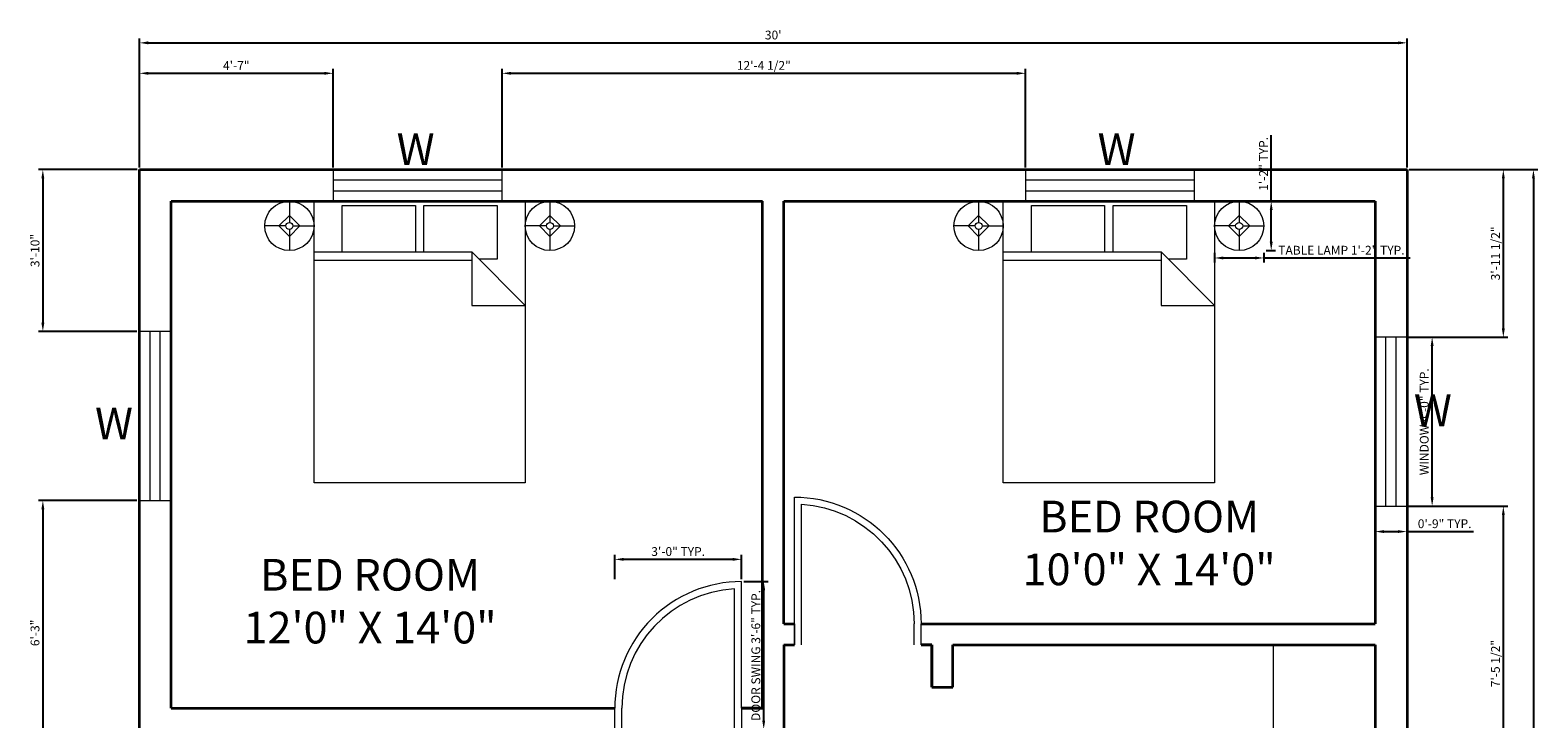
# Model space of a CAD drawing. Units: inches. Extents: x 1025 to 3479, y 1594 to 2212.
# Tile 6 of 9: x 2313 to 2741, y 1947 to 2142. Entities that reach past the tile are written whole.
import ezdxf

# ---------------------------------------------------------------- set-up
doc = ezdxf.new("R2010")
doc.units = ezdxf.units.IN
for name, color, linetype, lineweight in [('A-ANNO-DIMS', 1, 'Continuous', 18), ('A-ANNO-TEXT', 7, 'Continuous', 18), ('A-AREA-IDEN', 4, 'Continuous', 18), ('A-DOOR', 4, 'Continuous', 18), ('A-FLOR-CSWK', 8, 'Continuous', 18), ('A-FURN', 8, 'Continuous', 13), ('A-GLAZ', 3, 'Continuous', 18), ('A-WALL', 7, 'Continuous', 35)]:
    doc.layers.add(name, color=color, linetype=linetype, lineweight=lineweight)
doc.styles.get("Standard").update_dxf_attribs({"font": 'arial.ttf'})
doc.dimstyles.new('ISO-25', dxfattribs={"dimtxt": 2.5, "dimasz": 2.5, "dimexe": 1.25, "dimexo": 0.625, "dimtad": 1, "dimdec": 0, "dimlunit": 3, "dimtxsty": 'Standard', "dimcen": 2.5, "dimadec": 0, "dimazin": 0, "dimtfac": 1, "dimtdec": 0, "dimtmove": 0, "dimatfit": 3, "dimfxl": 1, "dimarcsym": 0})

# ---------------------------------------------------------------- blocks, each defined once
blk = doc.blocks.new('*D2')
at = {"layer": 'A-ANNO-DIMS', "color": 0, "lineweight": -2, "transparency": 16777216}
for p, q in [((2343.82, 2103.49), (2343.82, 2140.11)), ((2346.32, 2138.86), (2701.32, 2138.86)), ((2703.82, 2103.49), (2703.82, 2140.11))]:
    blk.add_line(p, q, dxfattribs=at)
at = {"layer": 'A-ANNO-DIMS', "color": 0, "transparency": 16777216}
for points in [[(2346.32, 2139.28), (2346.32, 2138.45), (2343.82, 2138.86)], [(2701.32, 2139.28), (2701.32, 2138.45), (2703.82, 2138.86)]]:
    blk.add_solid(points, dxfattribs=at)
at = {"layer": 'Defpoints', "color": 0, "transparency": 16777216}
for p in [(2703.82, 2138.86), (2343.82, 2102.86), (2703.82, 2102.86)]:
    blk.add_point(p, dxfattribs=at)
at = {"layer": 'A-ANNO-DIMS', "color": 0, "transparency": 16777216, "insert": (2523.82, 2140.76), "char_height": 2.5, "attachment_point": 5}
blk.add_mtext("30'", dxfattribs=at)
blk = doc.blocks.new('*D5')
at = {"layer": 'A-ANNO-DIMS', "color": 0, "lineweight": -2, "transparency": 16777216}
for p, q in [((2704.45, 2102.86), (2740.97, 2102.86)), ((2739.72, 2100.36), (2739.72, 1625.36)), ((2704.45, 1622.86), (2740.97, 1622.86))]:
    blk.add_line(p, q, dxfattribs=at)
at = {"layer": 'A-ANNO-DIMS', "color": 0, "transparency": 16777216}
for points in [[(2739.31, 2100.36), (2740.14, 2100.36), (2739.72, 2102.86)], [(2739.31, 1625.36), (2740.14, 1625.36), (2739.72, 1622.86)]]:
    blk.add_solid(points, dxfattribs=at)
at = {"layer": 'Defpoints', "color": 0, "transparency": 16777216}
for p in [(2703.82, 2102.86), (2703.82, 1622.86), (2739.72, 1622.86)]:
    blk.add_point(p, dxfattribs=at)
at = {"layer": 'A-ANNO-DIMS', "color": 0, "transparency": 16777216, "insert": (2737.82, 1862.86), "char_height": 2.5, "attachment_point": 5, "rotation": 90}
blk.add_mtext("40'", dxfattribs=at)
blk = doc.blocks.new('Bed - Queen')
for p, q in [((0, -80.00003), (0, 0)), ((0, 0), (59.99999, 0)), ((59.99999, 0), (59.99999, -80.00003)), ((7.99999, -1.2), (28.79998, -1.2)), ((7.99999, -14.4), (7.99999, -1.2)), ((28.79998, -1.2), (28.79998, -14.4)), ((31.19999, -1.2), (51.99999, -1.2)), ((31.19999, -14.4), (31.19999, -1.2)), ((51.99999, -1.2), (51.99999, -16.4)), ((0, -14.4), (44.8, -14.4)), ((44.8, -16.8), (0, -16.8)), ((59.99999, -29.6), (44.8, -14.4)), ((44.8, -14.4), (44.8, -29.6)), ((51.99999, -16.4), (46.79936, -16.4)), ((44.8, -29.6), (59.99999, -29.6)), ((59.99999, -80.00003), (0, -80.00003))]:
    blk.add_line(p, q)
blk = doc.blocks.new('Lamp - Table')
for p, q in [((0, 7), (0, 1)), ((-1, 0), (-7, 0)), ((0, 3), (-3, 0)), ((-3, 0), (0, -3)), ((3, 0), (0, 3)), ((0, -3), (3, 0)), ((1, 0), (7, 0)), ((0, -1), (0, -7))]:
    blk.add_line(p, q)
for radius in [7, 1]:
    blk.add_circle((0, 0), radius)
blk = doc.blocks.new('WIN-48IN')
for p, q in [((0, 48), (0, 0)), ((9, 48), (0, 48)), ((3, 48), (3, 0)), ((6, 0), (6, 48)), ((9, 0), (9, 48)), ((0, 0), (9, 0))]:
    blk.add_line(p, q)
blk = doc.blocks.new('DOOR-SWING-36IN')
for p, q in [((0, 36), (6, 36)), ((0, 34), (6, 34)), ((0, 2), (6, 2)), ((6, 0), (0, 0)), ((6, 2), (39.94, 2)), ((6, 0), (42, 0))]:
    blk.add_line(p, q)
for radius, start in [(36, 0), (34, 3.3723)]:
    blk.add_arc((6, 0), radius, start, 90)
blk = doc.blocks.new('*D20')
at = {"layer": 'A-ANNO-DIMS', "color": 0, "lineweight": -2, "transparency": 16777216}
for p, q in [((2704.38, 2055.25), (2712.2, 2055.25)), ((2710.95, 2009.75), (2710.95, 2052.75)), ((2704.38, 2007.25), (2712.2, 2007.25))]:
    blk.add_line(p, q, dxfattribs=at)
at = {"layer": 'A-ANNO-DIMS', "color": 0, "transparency": 16777216}
for points in [[(2710.54, 2052.75), (2711.37, 2052.75), (2710.95, 2055.25)], [(2710.54, 2009.75), (2711.37, 2009.75), (2710.95, 2007.25)]]:
    blk.add_solid(points, dxfattribs=at)
at = {"layer": 'Defpoints', "color": 0, "transparency": 16777216}
for p in [(2703.75, 2055.25), (2710.95, 2055.25), (2703.75, 2007.25)]:
    blk.add_point(p, dxfattribs=at)
at = {"layer": 'A-ANNO-DIMS', "color": 0, "transparency": 16777216, "insert": (2709.03, 2031.25), "char_height": 2.5, "attachment_point": 5, "rotation": 90}
blk.add_mtext('WINDOW 4\'-0" TYP.', dxfattribs=at)
blk = doc.blocks.new('*D21')
at = {"layer": 'A-ANNO-DIMS', "color": 0, "lineweight": -2, "transparency": 16777216}
for p, q in [((2694.75, 2006.63), (2694.75, 1998.8)), ((2703.75, 2006.63), (2703.75, 1998.8)), ((2697.25, 2000.05), (2701.25, 2000.05)), ((2703.75, 2000.05), (2722.74, 2000.05))]:
    blk.add_line(p, q, dxfattribs=at)
at = {"layer": 'A-ANNO-DIMS', "color": 0, "transparency": 16777216}
for points in [[(2697.25, 2000.47), (2697.25, 1999.64), (2694.75, 2000.05)], [(2701.25, 2000.47), (2701.25, 1999.64), (2703.75, 2000.05)]]:
    blk.add_solid(points, dxfattribs=at)
at = {"layer": 'Defpoints', "color": 0, "transparency": 16777216}
for p in [(2694.75, 2007.25), (2703.75, 2007.25), (2703.75, 2000.05)]:
    blk.add_point(p, dxfattribs=at)
at = {"layer": 'A-ANNO-DIMS', "color": 0, "transparency": 16777216, "insert": (2714.5, 2001.96), "char_height": 2.5, "attachment_point": 5}
blk.add_mtext('0\'-9" TYP.', dxfattribs=at)
blk = doc.blocks.new('*D26')
at = {"layer": 'A-ANNO-DIMS', "color": 0, "lineweight": -2, "transparency": 16777216}
for p, q in [((2649.15, 2079.24), (2649.15, 2076.51)), ((2651.65, 2077.76), (2660.65, 2077.76)), ((2663.15, 2079.24), (2663.15, 2076.51)), ((2663.15, 2077.76), (2704.72, 2077.76))]:
    blk.add_line(p, q, dxfattribs=at)
at = {"layer": 'A-ANNO-DIMS', "color": 0, "transparency": 16777216}
for points in [[(2651.65, 2078.18), (2651.65, 2077.35), (2649.15, 2077.76)], [(2660.65, 2078.18), (2660.65, 2077.35), (2663.15, 2077.76)]]:
    blk.add_solid(points, dxfattribs=at)
at = {"layer": 'Defpoints', "color": 0, "transparency": 16777216}
for p in [(2649.15, 2079.86), (2663.15, 2079.86), (2663.15, 2077.76)]:
    blk.add_point(p, dxfattribs=at)
at = {"layer": 'A-ANNO-DIMS', "color": 0, "transparency": 16777216, "insert": (2685.19, 2079.64), "char_height": 2.5, "attachment_point": 5}
blk.add_mtext('TABLE LAMP 1\'-2" TYP.', dxfattribs=at)
blk = doc.blocks.new('*D27')
at = {"layer": 'A-ANNO-DIMS', "color": 0, "lineweight": -2, "transparency": 16777216}
for p, q in [((2665.25, 2093.86), (2665.25, 2112.62)), ((2663.78, 2093.86), (2666.5, 2093.86)), ((2665.25, 2082.36), (2665.25, 2091.36)), ((2663.78, 2079.86), (2666.5, 2079.86))]:
    blk.add_line(p, q, dxfattribs=at)
at = {"layer": 'A-ANNO-DIMS', "color": 0, "transparency": 16777216}
for points in [[(2664.84, 2091.36), (2665.67, 2091.36), (2665.25, 2093.86)], [(2664.84, 2082.36), (2665.67, 2082.36), (2665.25, 2079.86)]]:
    blk.add_solid(points, dxfattribs=at)
at = {"layer": 'Defpoints', "color": 0, "transparency": 16777216}
for p in [(2663.15, 2093.86), (2665.25, 2093.86), (2663.15, 2079.86)]:
    blk.add_point(p, dxfattribs=at)
at = {"layer": 'A-ANNO-DIMS', "color": 0, "transparency": 16777216, "insert": (2663.37, 2104.49), "char_height": 2.5, "attachment_point": 5, "rotation": 90}
blk.add_mtext('1\'-2" TYP.', dxfattribs=at)
blk = doc.blocks.new('*D32')
at = {"layer": 'A-ANNO-DIMS', "color": 0, "lineweight": -2, "transparency": 16777216}
for p, q in [((2515.45, 1985.86), (2522.37, 1985.86)), ((2521.12, 1946.36), (2521.12, 1983.36)), ((2515.45, 1943.86), (2522.37, 1943.86))]:
    blk.add_line(p, q, dxfattribs=at)
at = {"layer": 'A-ANNO-DIMS', "color": 0, "transparency": 16777216}
for points in [[(2520.71, 1983.36), (2521.54, 1983.36), (2521.12, 1985.86)], [(2520.71, 1946.36), (2521.54, 1946.36), (2521.12, 1943.86)]]:
    blk.add_solid(points, dxfattribs=at)
at = {"layer": 'Defpoints', "color": 0, "transparency": 16777216}
for p in [(2514.82, 1985.86), (2521.12, 1985.86), (2514.82, 1943.86)]:
    blk.add_point(p, dxfattribs=at)
at = {"layer": 'A-ANNO-DIMS', "color": 0, "transparency": 16777216, "insert": (2519.2, 1964.86), "char_height": 2.5, "attachment_point": 5, "rotation": 90}
blk.add_mtext('DOOR SWING 3\'-6" TYP.', dxfattribs=at)
blk = doc.blocks.new('*D33')
at = {"layer": 'A-ANNO-DIMS', "color": 0, "lineweight": -2, "transparency": 16777216}
for p, q in [((2478.82, 1986.49), (2478.82, 1993.41)), ((2512.32, 1992.16), (2481.32, 1992.16)), ((2514.82, 1986.49), (2514.82, 1993.41))]:
    blk.add_line(p, q, dxfattribs=at)
at = {"layer": 'A-ANNO-DIMS', "color": 0, "transparency": 16777216}
for points in [[(2481.32, 1992.58), (2481.32, 1991.75), (2478.82, 1992.16)], [(2512.32, 1992.58), (2512.32, 1991.75), (2514.82, 1992.16)]]:
    blk.add_solid(points, dxfattribs=at)
at = {"layer": 'Defpoints', "color": 0, "transparency": 16777216}
for p in [(2478.82, 1992.16), (2478.82, 1985.86), (2514.82, 1985.86)]:
    blk.add_point(p, dxfattribs=at)
at = {"layer": 'A-ANNO-DIMS', "color": 0, "transparency": 16777216, "insert": (2496.82, 1994.06), "char_height": 2.5, "attachment_point": 5}
blk.add_mtext('3\'-0" TYP.', dxfattribs=at)
blk = doc.blocks.new('*D56')
at = {"layer": 'A-ANNO-DIMS', "color": 0, "lineweight": -2, "transparency": 16777216}
for p, q in [((2343.82, 2103.49), (2343.82, 2131.46)), ((2346.32, 2130.21), (2396.33, 2130.21)), ((2398.83, 2103.49), (2398.83, 2131.46))]:
    blk.add_line(p, q, dxfattribs=at)
at = {"layer": 'A-ANNO-DIMS', "color": 0, "transparency": 16777216}
for points in [[(2346.32, 2130.63), (2346.32, 2129.8), (2343.82, 2130.21)], [(2396.33, 2130.63), (2396.33, 2129.8), (2398.83, 2130.21)]]:
    blk.add_solid(points, dxfattribs=at)
at = {"layer": 'Defpoints', "color": 0, "transparency": 16777216}
for p in [(2398.83, 2130.21), (2343.82, 2102.86), (2398.83, 2102.86)]:
    blk.add_point(p, dxfattribs=at)
at = {"layer": 'A-ANNO-DIMS', "color": 0, "transparency": 16777216, "insert": (2371.33, 2132.09), "char_height": 2.5, "attachment_point": 5}
blk.add_mtext('4\'-7"', dxfattribs=at)
blk = doc.blocks.new('*D57')
at = {"layer": 'A-ANNO-DIMS', "color": 0, "lineweight": -2, "transparency": 16777216}
for p, q in [((2446.83, 2103.49), (2446.83, 2131.46)), ((2449.33, 2130.21), (2592.96, 2130.21)), ((2595.46, 2103.49), (2595.46, 2131.46))]:
    blk.add_line(p, q, dxfattribs=at)
at = {"layer": 'A-ANNO-DIMS', "color": 0, "transparency": 16777216}
for points in [[(2449.33, 2130.63), (2449.33, 2129.8), (2446.83, 2130.21)], [(2592.96, 2130.63), (2592.96, 2129.8), (2595.46, 2130.21)]]:
    blk.add_solid(points, dxfattribs=at)
at = {"layer": 'Defpoints', "color": 0, "transparency": 16777216}
for p in [(2595.46, 2130.21), (2446.83, 2102.86), (2595.46, 2102.86)]:
    blk.add_point(p, dxfattribs=at)
at = {"layer": 'A-ANNO-DIMS', "color": 0, "transparency": 16777216, "insert": (2521.15, 2132.13), "char_height": 2.5, "attachment_point": 5}
blk.add_mtext('12\'-4 1/2"', dxfattribs=at)
blk = doc.blocks.new('*D58')
at = {"layer": 'A-ANNO-DIMS', "color": 0, "lineweight": -2, "transparency": 16777216}
for p, q in [((2343.2, 2102.86), (2315.14, 2102.86)), ((2316.39, 2100.36), (2316.39, 2059.39)), ((2343.12, 2056.89), (2315.14, 2056.89))]:
    blk.add_line(p, q, dxfattribs=at)
at = {"layer": 'A-ANNO-DIMS', "color": 0, "transparency": 16777216}
for points in [[(2315.98, 2100.36), (2316.81, 2100.36), (2316.39, 2102.86)], [(2315.98, 2059.39), (2316.81, 2059.39), (2316.39, 2056.89)]]:
    blk.add_solid(points, dxfattribs=at)
at = {"layer": 'Defpoints', "color": 0, "transparency": 16777216}
for p in [(2343.82, 2102.86), (2316.39, 2056.89), (2343.74, 2056.89)]:
    blk.add_point(p, dxfattribs=at)
at = {"layer": 'A-ANNO-DIMS', "color": 0, "transparency": 16777216, "insert": (2314.49, 2079.88), "char_height": 2.5, "attachment_point": 5, "rotation": 90}
blk.add_mtext('3\'-10"', dxfattribs=at)
blk = doc.blocks.new('*D59')
at = {"layer": 'A-ANNO-DIMS', "color": 0, "lineweight": -2, "transparency": 16777216}
for p, q in [((2343.12, 2008.89), (2315.14, 2008.89)), ((2316.39, 2006.39), (2316.39, 1936.18)), ((2343.2, 1933.68), (2315.14, 1933.68))]:
    blk.add_line(p, q, dxfattribs=at)
at = {"layer": 'A-ANNO-DIMS', "color": 0, "transparency": 16777216}
for points in [[(2315.98, 2006.39), (2316.81, 2006.39), (2316.39, 2008.89)], [(2315.98, 1936.18), (2316.81, 1936.18), (2316.39, 1933.68)]]:
    blk.add_solid(points, dxfattribs=at)
at = {"layer": 'Defpoints', "color": 0, "transparency": 16777216}
for p in [(2343.74, 2008.89), (2316.39, 1933.68), (2343.82, 1933.68)]:
    blk.add_point(p, dxfattribs=at)
at = {"layer": 'A-ANNO-DIMS', "color": 0, "transparency": 16777216, "insert": (2314.49, 1971.28), "char_height": 2.5, "attachment_point": 5, "rotation": 90}
blk.add_mtext('6\'-3"', dxfattribs=at)
blk = doc.blocks.new('*D74')
at = {"layer": 'A-ANNO-DIMS', "color": 0, "lineweight": -2, "transparency": 16777216}
for p, q in [((2704.45, 2102.86), (2732.42, 2102.86)), ((2731.17, 2100.36), (2731.17, 2057.75)), ((2704.38, 2055.25), (2732.42, 2055.25))]:
    blk.add_line(p, q, dxfattribs=at)
at = {"layer": 'A-ANNO-DIMS', "color": 0, "transparency": 16777216}
for points in [[(2730.76, 2100.36), (2731.59, 2100.36), (2731.17, 2102.86)], [(2730.76, 2057.75), (2731.59, 2057.75), (2731.17, 2055.25)]]:
    blk.add_solid(points, dxfattribs=at)
at = {"layer": 'Defpoints', "color": 0, "transparency": 16777216}
for p in [(2703.82, 2102.86), (2703.75, 2055.25), (2731.17, 2055.25)]:
    blk.add_point(p, dxfattribs=at)
at = {"layer": 'A-ANNO-DIMS', "color": 0, "transparency": 16777216, "insert": (2729.26, 2079.06), "char_height": 2.5, "attachment_point": 5, "rotation": 90}
blk.add_mtext('3\'-11 1/2"', dxfattribs=at)
blk = doc.blocks.new('*D75')
at = {"layer": 'A-ANNO-DIMS', "color": 0, "lineweight": -2, "transparency": 16777216}
for p, q in [((2704.38, 2007.25), (2732.42, 2007.25)), ((2731.17, 2004.75), (2731.17, 1920.36)), ((2704.35, 1917.86), (2732.42, 1917.86))]:
    blk.add_line(p, q, dxfattribs=at)
at = {"layer": 'A-ANNO-DIMS', "color": 0, "transparency": 16777216}
for points in [[(2730.76, 2004.75), (2731.59, 2004.75), (2731.17, 2007.25)], [(2730.76, 1920.36), (2731.59, 1920.36), (2731.17, 1917.86)]]:
    blk.add_solid(points, dxfattribs=at)
at = {"layer": 'Defpoints', "color": 0, "transparency": 16777216}
for p in [(2703.75, 2007.25), (2703.72, 1917.86), (2731.17, 1917.86)]:
    blk.add_point(p, dxfattribs=at)
at = {"layer": 'A-ANNO-DIMS', "color": 0, "transparency": 16777216, "insert": (2729.26, 1962.56), "char_height": 2.5, "attachment_point": 5, "rotation": 90}
blk.add_mtext('7\'-5 1/2"', dxfattribs=at)

msp = doc.modelspace()

# ---------------------------------------------------------------- linework, layer by layer
at = {"layer": 'A-DOOR'}
for p, q in [((2512.82, 1985.81), (2512.82, 1985.86)), ((2529.82, 1967.86), (2529.82, 1973.86))]:
    msp.add_line(p, q, dxfattribs=at)
at = {"layer": 'A-FLOR-CSWK'}
msp.add_line((2665.82, 1967.86), (2665.82, 1852.86), dxfattribs=at)
at = {"layer": 'A-WALL'}
for p, q in [((2343.82, 2102.86), (2703.82, 2102.86)), ((2343.82, 1622.86), (2343.82, 2102.86)), ((2703.82, 2102.86), (2703.82, 1622.86)), ((2352.82, 2093.86), (2520.82, 2093.86)), ((2352.82, 1949.86), (2352.82, 2093.86)), ((2520.82, 1949.86), (2520.82, 2093.86)), ((2526.82, 1973.86), (2526.82, 2093.86)), ((2526.82, 2093.86), (2694.82, 2093.86)), ((2694.82, 2093.86), (2694.82, 1973.86)), ((2526.82, 1973.86), (2529.82, 1973.86)), ((2565.82, 1973.86), (2694.82, 1973.86)), ((2526.82, 1967.86), (2529.82, 1967.86)), ((2526.82, 1967.86), (2526.82, 1943.86)), ((2568.82, 1967.86), (2565.82, 1967.86)), ((2565.82, 1967.86), (2568.82, 1967.86)), ((2568.82, 1967.86), (2568.82, 1955.86)), ((2568.82, 1955.86), (2568.82, 1967.86)), ((2574.82, 1967.86), (2694.82, 1967.86)), ((2574.82, 1955.86), (2574.82, 1967.86)), ((2694.82, 1967.86), (2694.82, 1823.86)), ((2568.82, 1955.86), (2574.82, 1955.86)), ((2352.82, 1949.86), (2478.82, 1949.86)), ((2520.82, 1949.86), (2514.82, 1949.86)), ((2514.82, 1949.86), (2520.82, 1949.86))]:
    msp.add_line(p, q, dxfattribs=at)

# ---------------------------------------------------------------- block references
at = {"layer": 'A-DOOR', "extrusion": (0, 0, -1), "zscale": -1, "rotation": 90.0000000000004}
msp.add_blockref('DOOR-SWING-36IN', (-2529.82, 1967.86), dxfattribs=at)
at = {"layer": 'A-DOOR', "rotation": 89.99999999999888}
msp.add_blockref('DOOR-SWING-36IN', (2514.82, 1943.86), dxfattribs=at)
at = {"layer": 'A-FURN'}
for name, p in [('Lamp - Table', (2386.41, 2086.86)), ('Bed - Queen', (2393.41, 2093.86)), ('Lamp - Table', (2460.41, 2086.86)), ('Lamp - Table', (2582.15, 2086.86)), ('Bed - Queen', (2589.15, 2093.86)), ('Lamp - Table', (2656.15, 2086.86))]:
    msp.add_blockref(name, p, dxfattribs=at)
at = {"layer": 'A-GLAZ', "rotation": 270.0000000000019}
for p in [(2398.83, 2102.86), (2595.46, 2102.86)]:
    msp.add_blockref('WIN-48IN', p, dxfattribs=at)
at = {"layer": 'A-GLAZ'}
for p in [(2343.74, 2008.89), (2694.75, 2007.25)]:
    msp.add_blockref('WIN-48IN', p, dxfattribs=at)

# ---------------------------------------------------------------- texts
at = {"layer": 'A-ANNO-TEXT', "char_height": 9, "attachment_point": 1}
for insert in [(2414.33, 2113.13), (2613.4, 2113.16), (2703.22, 2038.99), (2328.66, 2035.27)]:
    msp.add_mtext_dynamic_manual_height_columns('\\pxqc;W', width=15.8719, gutter_width=12.5, heights=[0], dxfattribs=dict(at, insert=insert))
at = {"layer": 'A-AREA-IDEN', "char_height": 9, "attachment_point": 1}
for s, heights, insert in [('\\pxqc;BED ROOM \\P10\'0" X 14\'0"', [0], (2583.97, 2008.82)), ('\\pxqc;BED ROOM \\P12\'0" X 14\'0"', [24.35], (2362.72, 1992.28))]:
    msp.add_mtext_dynamic_manual_height_columns(s, width=93.2353, gutter_width=12.5, heights=heights, dxfattribs=dict(at, insert=insert))

# ---------------------------------------------------------------- dimensions: what is measured, and where the dimension line sits
at = {"layer": 'A-ANNO-DIMS'}
for base, p1, p2, override, picture, middle in [((2703.82, 2138.86), (2343.82, 2102.86), (2703.82, 2102.86), {"dimclrd": 0, "dimclre": 0, "dimclrt": 0}, '*D2', (2523.82, 2140.76)), ((2398.83, 2130.21), (2343.82, 2102.86), (2398.83, 2102.86), {"dimdec": 1, "dimlfac": 1, "dimrnd": 0, "dimzin": 1, "dimdsep": 46, "dimlunit": 4, "dimfrac": 2}, '*D56', (2371.33, 2132.09)), ((2595.46, 2130.21), (2446.83, 2102.86), (2595.46, 2102.86), {"dimdec": 1, "dimlfac": 1, "dimrnd": 0, "dimzin": 1, "dimdsep": 46, "dimlunit": 4, "dimfrac": 2}, '*D57', (2521.15, 2132.13))]:
    dim = msp.add_linear_dim(base=base, p1=p1, p2=p2, dimstyle='ISO-25', override=override, dxfattribs=at)
    dim.commit()
    dim.dimension.update_dxf_attribs({"geometry": picture, "text_midpoint": middle})
for base, p1, p2, angle, text, picture, middle in [((2665.25, 2093.86), (2663.15, 2079.86), (2663.15, 2093.86), 90, '<> TYP.', '*D27', (2663.37, 2104.49)), ((2710.95, 2055.25), (2703.75, 2007.25), (2703.75, 2055.25), 90, 'WINDOW <> TYP.', '*D20', (2709.03, 2031.25)), ((2478.82, 1992.16), (2514.82, 1985.86), (2478.82, 1985.86), 180, '<> TYP.', '*D33', (2496.82, 1994.06)), ((2521.12, 1985.86), (2514.82, 1943.86), (2514.82, 1985.86), 90, 'DOOR SWING <> TYP.', '*D32', (2519.2, 1964.86))]:
    dim = msp.add_linear_dim(base=base, p1=p1, p2=p2, angle=angle, text=text, dimstyle='ISO-25', override={"dimdec": 1, "dimlfac": 1, "dimrnd": 0, "dimzin": 1, "dimdsep": 46, "dimlunit": 4, "dimfrac": 2}, dxfattribs=at)
    dim.commit()
    dim.dimension.update_dxf_attribs({"geometry": picture, "text_midpoint": middle})
for base, p1, p2, override, picture, middle in [((2316.39, 2056.89), (2343.82, 2102.86), (2343.74, 2056.89), {"dimdec": 1, "dimlfac": 1, "dimrnd": 0, "dimzin": 1, "dimdsep": 46, "dimlunit": 4, "dimfrac": 2}, '*D58', (2314.49, 2079.88)), ((2731.17, 2055.25), (2703.82, 2102.86), (2703.75, 2055.25), {"dimdec": 1, "dimlfac": 1, "dimrnd": 0, "dimzin": 1, "dimdsep": 46, "dimlunit": 4, "dimfrac": 2}, '*D74', (2729.26, 2079.06)), ((2739.72, 1622.86), (2703.82, 2102.86), (2703.82, 1622.86), {"dimclrd": 0, "dimclre": 0, "dimclrt": 0}, '*D5', (2737.82, 1862.86)), ((2316.39, 1933.68), (2343.74, 2008.89), (2343.82, 1933.68), {"dimdec": 1, "dimlfac": 1, "dimrnd": 0, "dimzin": 1, "dimdsep": 46, "dimlunit": 4, "dimfrac": 2}, '*D59', (2314.49, 1971.28)), ((2731.17, 1917.86), (2703.75, 2007.25), (2703.72, 1917.86), {"dimdec": 1, "dimlfac": 1, "dimrnd": 0, "dimzin": 1, "dimdsep": 46, "dimlunit": 4, "dimfrac": 2}, '*D75', (2729.26, 1962.56))]:
    dim = msp.add_linear_dim(base=base, p1=p1, p2=p2, angle=90, dimstyle='ISO-25', override=override, dxfattribs=at)
    dim.commit()
    dim.dimension.update_dxf_attribs({"geometry": picture, "text_midpoint": middle})
for base, p1, p2, text, picture, middle in [((2663.15, 2077.76), (2649.15, 2079.86), (2663.15, 2079.86), 'TABLE LAMP <> TYP.', '*D26', (2685.19, 2079.64)), ((2703.75, 2000.05), (2694.75, 2007.25), (2703.75, 2007.25), '<> TYP.', '*D21', (2714.5, 2001.96))]:
    dim = msp.add_linear_dim(base=base, p1=p1, p2=p2, text=text, dimstyle='ISO-25', override={"dimdec": 1, "dimlfac": 1, "dimrnd": 0, "dimzin": 1, "dimdsep": 46, "dimlunit": 4, "dimfrac": 2}, dxfattribs=at)
    dim.commit()
    dim.dimension.update_dxf_attribs({"geometry": picture, "text_midpoint": middle})

doc.saveas('drawing.dxf')
